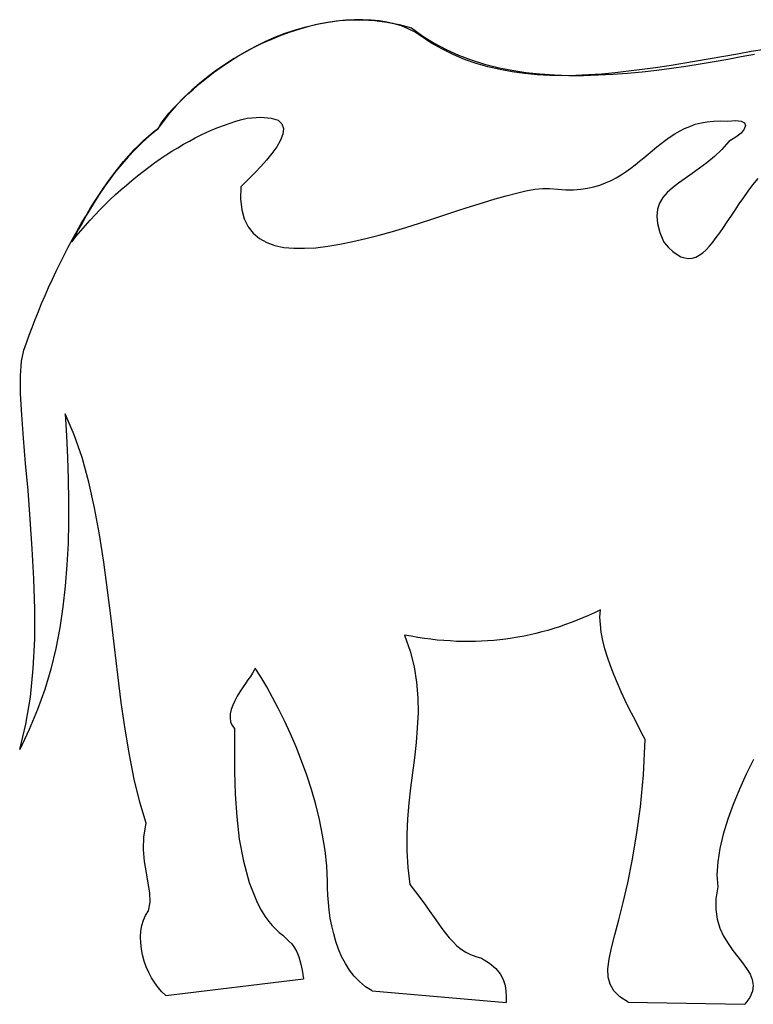
# Model space of a CAD drawing. Units: inches. Extents: x 386 to 107067, y -7 to 96314.
# Tile 9 of 10: x 107062.699 to 107064.862, y 96311.382 to 96314.283. Entities that reach past the tile are written whole.
import ezdxf

# ---------------------------------------------------------------- set-up
doc = ezdxf.new("R2010")
doc.units = ezdxf.units.IN
doc.layers.add('A-ELEV', color=7, linetype='Continuous', lineweight=25)
doc.layers.add('freecads.com', color=7, linetype='Continuous')

# ---------------------------------------------------------------- blocks, each defined once
blk = doc.blocks.new('elephant')
at = {"layer": 'freecads.com'}
for p, q in [((104457.3165, 95264.9791), (104457.3504, 95264.9835)), ((104457.3684, 95264.9845), (104457.3416, 95264.9818)), ((104457.3504, 95264.9835), (104457.3843, 95264.9856)), ((104457.3941, 95264.9862), (104457.3684, 95264.9845)), ((104457.3843, 95264.9856), (104457.4193, 95264.9856)), ((104457.4193, 95264.9862), (104457.3941, 95264.9862)), ((104457.4439, 95264.9851), (104457.4193, 95264.9862)), ((104457.4193, 95264.9856), (104457.4543, 95264.9835)), ((104457.4674, 95264.9829), (104457.4439, 95264.9851)), ((104457.4543, 95264.9835), (104457.4898, 95264.9791)), ((104457.4898, 95264.9791), (104457.4674, 95264.9829)), ((104457.1896, 95264.9463), (104457.2202, 95264.9567)), ((104457.2328, 95264.9583), (104457.2049, 95264.949)), ((104457.2202, 95264.9567), (104457.2514, 95264.9654)), ((104457.2601, 95264.966), (104457.2328, 95264.9583)), ((104457.2514, 95264.9654), (104457.2836, 95264.9731)), ((104457.288, 95264.9725), (104457.2601, 95264.966)), ((104457.2836, 95264.9731), (104457.3165, 95264.9791)), ((104457.3148, 95264.9774), (104457.288, 95264.9725)), ((104457.3416, 95264.9818), (104457.3148, 95264.9774)), ((104457.4898, 95264.9791), (104457.5259, 95264.972)), ((104457.5117, 95264.9742), (104457.4898, 95264.9791)), ((104457.5325, 95264.9676), (104457.5117, 95264.9742)), ((104457.5259, 95264.972), (104457.5625, 95264.9621)), ((104457.5522, 95264.9594), (104457.5325, 95264.9676)), ((104457.5708, 95264.9501), (104457.5522, 95264.9594)), ((104457.5625, 95264.9621), (104457.5954, 95264.9381)), ((104457.1491, 95264.9277), (104457.1212, 95264.9156)), ((104457.1311, 95264.9217), (104457.1595, 95264.9342)), ((104457.177, 95264.9392), (104457.1491, 95264.9277)), ((104457.1595, 95264.9342), (104457.1896, 95264.9463)), ((104457.2049, 95264.949), (104457.177, 95264.9392)), ((104457.5877, 95264.9392), (104457.5708, 95264.9501)), ((104457.6194, 95264.9184), (104457.5877, 95264.9392)), ((104457.5954, 95264.9381), (104457.6292, 95264.9167)), ((104457.0939, 95264.902), (104457.0665, 95264.8872)), ((104457.0758, 95264.8932), (104457.1032, 95264.908)), ((104457.1212, 95264.9156), (104457.0939, 95264.902)), ((104457.1032, 95264.908), (104457.1311, 95264.9217)), ((104457.6517, 95264.8998), (104457.6194, 95264.9184)), ((104457.6292, 95264.9167), (104457.6648, 95264.8981)), ((104457.685, 95264.8834), (104457.6517, 95264.8998)), ((104457.6648, 95264.8981), (104457.7009, 95264.8817)), ((104458.6048, 95264.8987), (104458.5644, 95264.8921)), ((104457.0398, 95264.8719), (104457.0135, 95264.8549)), ((104457.0255, 95264.8626), (104457.0501, 95264.8784)), ((104457.0665, 95264.8872), (104457.0398, 95264.8719)), ((104457.0501, 95264.8784), (104457.0758, 95264.8932)), ((104457.7184, 95264.8691), (104457.685, 95264.8834)), ((104457.7009, 95264.8817), (104457.7386, 95264.8675)), ((104457.7528, 95264.8571), (104457.7184, 95264.8691)), ((104457.7386, 95264.8675), (104457.7775, 95264.8555)), ((104458.443, 95264.8708), (104458.4025, 95264.8642)), ((104458.4834, 95264.8779), (104458.443, 95264.8708)), ((104458.4545, 95264.8631), (104458.4949, 95264.8702)), ((104458.5239, 95264.885), (104458.4834, 95264.8779)), ((104458.4949, 95264.8702), (104458.5348, 95264.8773)), ((104458.5644, 95264.8921), (104458.5239, 95264.885)), ((104458.5348, 95264.8773), (104458.5737, 95264.885)), ((104456.9878, 95264.8374), (104456.9626, 95264.8189)), ((104456.979, 95264.8303), (104457.0015, 95264.8467)), ((104457.0135, 95264.8549), (104456.9878, 95264.8374)), ((104457.0015, 95264.8467), (104457.0255, 95264.8626)), ((104457.7878, 95264.8473), (104457.7528, 95264.8571)), ((104457.7775, 95264.8555), (104457.8174, 95264.8451)), ((104457.8234, 95264.8391), (104457.7878, 95264.8473)), ((104457.8174, 95264.8451), (104457.8579, 95264.8374)), ((104457.8595, 95264.8325), (104457.8234, 95264.8391)), ((104457.8579, 95264.8374), (104457.8994, 95264.8309)), ((104458.2423, 95264.8391), (104458.2024, 95264.8342)), ((104458.2822, 95264.8446), (104458.2423, 95264.8391)), ((104458.2429, 95264.8325), (104458.286, 95264.8374)), ((104458.3221, 95264.8506), (104458.2822, 95264.8446)), ((104458.286, 95264.8374), (104458.3287, 95264.8435)), ((104458.3621, 95264.8571), (104458.3221, 95264.8506)), ((104458.3287, 95264.8435), (104458.3714, 95264.8495)), ((104458.4025, 95264.8642), (104458.3621, 95264.8571)), ((104458.3714, 95264.8495), (104458.4135, 95264.856)), ((104458.4135, 95264.856), (104458.4545, 95264.8631)), ((104456.9626, 95264.8189), (104456.938, 95264.7992)), ((104456.938, 95264.7981), (104456.9577, 95264.8139)), ((104456.9577, 95264.8139), (104456.979, 95264.8303)), ((104457.8961, 95264.8276), (104457.8595, 95264.8325)), ((104457.9328, 95264.8238), (104457.8961, 95264.8276)), ((104457.8994, 95264.8309), (104457.941, 95264.8265)), ((104457.9705, 95264.8221), (104457.9328, 95264.8238)), ((104457.941, 95264.8265), (104457.9836, 95264.8232)), ((104458.0082, 95264.821), (104457.9705, 95264.8221)), ((104457.9836, 95264.8232), (104458.0263, 95264.8221)), ((104458.0465, 95264.8216), (104458.0082, 95264.821)), ((104458.0263, 95264.8221), (104458.0695, 95264.8221)), ((104458.0848, 95264.8232), (104458.0465, 95264.8216)), ((104458.0695, 95264.8221), (104458.1127, 95264.8232)), ((104458.1236, 95264.826), (104458.0848, 95264.8232)), ((104458.1127, 95264.8232), (104458.1559, 95264.8254)), ((104458.163, 95264.8298), (104458.1236, 95264.826)), ((104458.1559, 95264.8254), (104458.1996, 95264.8287)), ((104458.2024, 95264.8342), (104458.163, 95264.8298)), ((104458.1996, 95264.8287), (104458.2429, 95264.8325)), ((104456.9019, 95264.7663), (104456.9194, 95264.7817)), ((104456.938, 95264.7992), (104456.9145, 95264.7784)), ((104456.9194, 95264.7817), (104456.938, 95264.7981)), ((104456.8915, 95264.757), (104456.8697, 95264.7341)), ((104456.8719, 95264.7368), (104456.8861, 95264.751)), ((104456.8861, 95264.751), (104456.9019, 95264.7663)), ((104456.9145, 95264.7784), (104456.8915, 95264.757)), ((104456.8472, 95264.7106), (104456.8587, 95264.7231)), ((104456.8697, 95264.7341), (104456.8489, 95264.7111)), ((104456.8587, 95264.7231), (104456.8719, 95264.7368)), ((104456.8489, 95264.7111), (104456.8297, 95264.6865)), ((104456.8297, 95264.6887), (104456.8379, 95264.6985)), ((104456.8379, 95264.6985), (104456.8472, 95264.7106)), ((104457.0447, 95264.6871), (104457.0616, 95264.692)), ((104457.0616, 95264.692), (104457.078, 95264.6958)), ((104457.078, 95264.6958), (104457.1185, 95264.6985)), ((104457.1185, 95264.6985), (104457.1486, 95264.6964)), ((104457.1486, 95264.6964), (104457.1688, 95264.6898)), ((104456.8013, 95264.6553), (104456.8161, 95264.6663)), ((104456.8297, 95264.6865), (104456.8111, 95264.6613)), ((104456.8161, 95264.6663), (104456.8188, 95264.6723)), ((104456.8188, 95264.6723), (104456.8232, 95264.6794)), ((104456.8232, 95264.6794), (104456.8297, 95264.6887)), ((104456.9768, 95264.6624), (104456.9938, 95264.6696)), ((104456.9938, 95264.6696), (104457.0108, 95264.6756)), ((104457.0108, 95264.6756), (104457.0277, 95264.6816)), ((104457.0277, 95264.6816), (104457.0447, 95264.6871)), ((104457.1688, 95264.6898), (104457.1803, 95264.6794)), ((104457.1803, 95264.6794), (104457.1852, 95264.6652)), ((104457.1852, 95264.6652), (104457.183, 95264.6493)), ((104458.3528, 95264.6581), (104458.3675, 95264.6652)), ((104458.3675, 95264.6652), (104458.3828, 95264.6717)), ((104458.3828, 95264.6717), (104458.3993, 95264.6778)), ((104458.3993, 95264.6778), (104458.4162, 95264.6821)), ((104458.4162, 95264.6821), (104458.4342, 95264.6854)), ((104458.4342, 95264.6854), (104458.4534, 95264.6876)), ((104458.4534, 95264.6876), (104458.473, 95264.6882)), ((104458.473, 95264.6882), (104458.4944, 95264.6871)), ((104458.4944, 95264.6871), (104458.5184, 95264.6892)), ((104458.5184, 95264.6892), (104458.5348, 95264.6876)), ((104458.5436, 95264.6635), (104458.5343, 95264.652)), ((104458.5348, 95264.6876), (104458.5447, 95264.6821)), ((104458.5474, 95264.6739), (104458.5436, 95264.6635)), ((104458.5447, 95264.6821), (104458.5474, 95264.6739)), ((104456.7887, 95264.6428), (104456.7669, 95264.6231)), ((104456.7718, 95264.6302), (104456.7865, 95264.6433)), ((104456.7865, 95264.6433), (104456.8013, 95264.6553)), ((104456.8111, 95264.6613), (104456.7887, 95264.6428)), ((104456.9074, 95264.6285), (104456.9249, 95264.6378)), ((104456.9249, 95264.6378), (104456.9424, 95264.6466)), ((104456.9424, 95264.6466), (104456.9593, 95264.6548)), ((104456.9593, 95264.6548), (104456.9768, 95264.6624)), ((104457.183, 95264.6493), (104457.1765, 95264.6313)), ((104458.3117, 95264.6313), (104458.3249, 95264.6411)), ((104458.3249, 95264.6411), (104458.3385, 95264.6499)), ((104458.3385, 95264.6499), (104458.3528, 95264.6581)), ((104458.5184, 95264.6395), (104458.4977, 95264.6274)), ((104458.5343, 95264.652), (104458.5184, 95264.6395)), ((104456.7422, 95264.6012), (104456.757, 95264.6159)), ((104456.7669, 95264.6231), (104456.7466, 95264.6028)), ((104456.757, 95264.6159), (104456.7718, 95264.6302)), ((104456.8554, 95264.5985), (104456.8729, 95264.6088)), ((104456.8729, 95264.6088), (104456.8905, 95264.6192)), ((104456.8905, 95264.6192), (104456.9074, 95264.6285)), ((104457.165, 95264.6116), (104457.1508, 95264.5919)), ((104457.1765, 95264.6313), (104457.165, 95264.6116)), ((104458.2729, 95264.6006), (104458.2855, 95264.611)), ((104458.2855, 95264.611), (104458.2986, 95264.6214)), ((104458.2986, 95264.6214), (104458.3117, 95264.6313)), ((104458.4977, 95264.6274), (104458.4774, 95264.6039)), ((104456.7269, 95264.5821), (104456.7083, 95264.5607)), ((104456.7133, 95264.5684), (104456.728, 95264.5848)), ((104456.7466, 95264.6028), (104456.7269, 95264.5821)), ((104456.728, 95264.5848), (104456.7422, 95264.6012)), ((104456.8046, 95264.564), (104456.8215, 95264.576)), ((104456.8215, 95264.576), (104456.8385, 95264.5875)), ((104456.8385, 95264.5875), (104456.8554, 95264.5985)), ((104457.1508, 95264.5919), (104457.1349, 95264.5722)), ((104458.2352, 95264.5689), (104458.2478, 95264.5793)), ((104458.2478, 95264.5793), (104458.2604, 95264.5903)), ((104458.2604, 95264.5903), (104458.2729, 95264.6006)), ((104458.4561, 95264.5831), (104458.4337, 95264.5646)), ((104458.4774, 95264.6039), (104458.4561, 95264.5831)), ((104456.6848, 95264.5317), (104456.699, 95264.5503)), ((104456.7083, 95264.5607), (104456.6908, 95264.5394)), ((104456.699, 95264.5503), (104456.7133, 95264.5684)), ((104456.7707, 95264.5389), (104456.7876, 95264.5514)), ((104456.7876, 95264.5514), (104456.8046, 95264.564)), ((104457.1179, 95264.5531), (104457.1015, 95264.5361)), ((104457.1349, 95264.5722), (104457.1179, 95264.5531)), ((104458.1953, 95264.5383), (104458.2089, 95264.5482)), ((104458.2089, 95264.5482), (104458.2221, 95264.5585)), ((104458.2221, 95264.5585), (104458.2352, 95264.5689)), ((104458.4118, 95264.5482), (104458.3905, 95264.5328)), ((104458.4337, 95264.5646), (104458.4118, 95264.5482)), ((104456.6701, 95264.5126), (104456.6848, 95264.5317)), ((104456.6908, 95264.5394), (104456.6739, 95264.5175)), ((104456.7379, 95264.5126), (104456.7543, 95264.5263)), ((104456.7543, 95264.5263), (104456.7707, 95264.5389)), ((104457.0862, 95264.5208), (104457.0736, 95264.5082)), ((104457.1015, 95264.5361), (104457.0862, 95264.5208)), ((104458.151, 95264.5126), (104458.1663, 95264.5203)), ((104458.1663, 95264.5203), (104458.181, 95264.529)), ((104458.181, 95264.529), (104458.1953, 95264.5383)), ((104458.3697, 95264.5186), (104458.35, 95264.5044)), ((104458.3905, 95264.5328), (104458.3697, 95264.5186)), ((104458.5693, 95264.4995), (104458.5846, 95264.5181)), ((104456.6422, 95264.4721), (104456.6564, 95264.4929)), ((104456.658, 95264.4956), (104456.6433, 95264.4738)), ((104456.6564, 95264.4929), (104456.6701, 95264.5126)), ((104456.6739, 95264.5175), (104456.658, 95264.4956)), ((104456.7056, 95264.4852), (104456.7215, 95264.4989)), ((104456.7215, 95264.4989), (104456.7379, 95264.5126)), ((104457.0594, 95264.494), (104457.0583, 95264.4579)), ((104457.0643, 95264.4989), (104457.0594, 95264.494)), ((104457.0736, 95264.5082), (104457.0643, 95264.4989)), ((104457.9257, 95264.4863), (104457.9486, 95264.4891)), ((104457.9486, 95264.4891), (104457.9689, 95264.4891)), ((104457.9689, 95264.4891), (104457.994, 95264.4863)), ((104458.0613, 95264.4863), (104458.081, 95264.4896)), ((104458.081, 95264.4896), (104458.1001, 95264.4935)), ((104458.1001, 95264.4935), (104458.1176, 95264.4989)), ((104458.1176, 95264.4989), (104458.1346, 95264.5055)), ((104458.1346, 95264.5055), (104458.151, 95264.5126)), ((104458.3325, 95264.4907), (104458.3167, 95264.4765)), ((104458.35, 95264.5044), (104458.3325, 95264.4907)), ((104458.5551, 95264.4809), (104458.5693, 95264.4995)), ((104456.6285, 95264.4513), (104456.6422, 95264.4721)), ((104456.6433, 95264.4738), (104456.6291, 95264.4519)), ((104456.6739, 95264.4563), (104456.6897, 95264.471)), ((104456.6897, 95264.471), (104456.7056, 95264.4852)), ((104457.8092, 95264.4579), (104457.8415, 95264.4672)), ((104457.8415, 95264.4672), (104457.8721, 95264.4754)), ((104457.8721, 95264.4754), (104457.8999, 95264.482)), ((104457.8999, 95264.482), (104457.9257, 95264.4863)), ((104457.994, 95264.4863), (104458.0175, 95264.4847)), ((104458.0175, 95264.4847), (104458.0399, 95264.4847)), ((104458.0399, 95264.4847), (104458.0613, 95264.4863)), ((104458.3035, 95264.4617), (104458.2937, 95264.4459)), ((104458.3167, 95264.4765), (104458.3035, 95264.4617)), ((104458.5288, 95264.4437), (104458.542, 95264.4623)), ((104458.542, 95264.4623), (104458.5551, 95264.4809)), ((104456.6148, 95264.4295), (104456.6285, 95264.4513)), ((104456.6291, 95264.4519), (104456.6159, 95264.43)), ((104456.6438, 95264.4262), (104456.6586, 95264.4415)), ((104456.6586, 95264.4415), (104456.6739, 95264.4563)), ((104457.0583, 95264.4579), (104457.0622, 95264.4262)), ((104457.702, 95264.4246), (104457.7392, 95264.4366)), ((104457.7392, 95264.4366), (104457.7747, 95264.4475)), ((104457.7747, 95264.4475), (104457.8092, 95264.4579)), ((104458.2937, 95264.4459), (104458.2877, 95264.4278)), ((104458.5168, 95264.4251), (104458.5288, 95264.4437)), ((104456.5886, 95264.3852), (104456.6017, 95264.4076)), ((104456.6033, 95264.4092), (104456.5919, 95264.3885)), ((104456.6017, 95264.4076), (104456.6148, 95264.4295)), ((104456.6159, 95264.43), (104456.6033, 95264.4092)), ((104456.6148, 95264.3956), (104456.6291, 95264.4109)), ((104456.6291, 95264.4109), (104456.6438, 95264.4262)), ((104457.0622, 95264.4262), (104457.0693, 95264.3989)), ((104457.6249, 95264.3994), (104457.6637, 95264.412)), ((104457.6637, 95264.412), (104457.702, 95264.4246)), ((104458.2877, 95264.4278), (104458.2855, 95264.4076)), ((104458.2855, 95264.4076), (104458.2877, 95264.3852)), ((104458.4933, 95264.3907), (104458.5048, 95264.4076)), ((104458.5048, 95264.4076), (104458.5168, 95264.4251)), ((104456.5754, 95264.3622), (104456.5886, 95264.3852)), ((104456.5919, 95264.3885), (104456.5809, 95264.3688)), ((104456.5869, 95264.3638), (104456.6006, 95264.3797)), ((104456.6006, 95264.3797), (104456.6148, 95264.3956)), ((104457.0693, 95264.3989), (104457.0807, 95264.3759)), ((104457.0807, 95264.3759), (104457.0955, 95264.3567)), ((104457.5062, 95264.3622), (104457.5461, 95264.3742)), ((104457.5461, 95264.3742), (104457.5855, 95264.3868)), ((104457.5855, 95264.3868), (104457.6249, 95264.3994)), ((104458.2877, 95264.3852), (104458.2942, 95264.3595)), ((104458.4714, 95264.3584), (104458.4823, 95264.3742)), ((104458.4823, 95264.3742), (104458.4933, 95264.3907)), ((104456.5705, 95264.3496), (104456.5607, 95264.3316)), ((104456.5607, 95264.3316), (104456.5738, 95264.348)), ((104456.5629, 95264.3392), (104456.5754, 95264.3622)), ((104456.5809, 95264.3688), (104456.5705, 95264.3496)), ((104456.5738, 95264.348), (104456.5869, 95264.3638)), ((104457.0955, 95264.3567), (104457.1141, 95264.3414)), ((104457.4275, 95264.3409), (104457.4668, 95264.3513)), ((104457.4668, 95264.3513), (104457.5062, 95264.3622)), ((104458.2942, 95264.3595), (104458.3068, 95264.3305)), ((104458.4512, 95264.3305), (104458.461, 95264.3442)), ((104458.461, 95264.3442), (104458.4714, 95264.3584)), ((104456.5383, 95264.2922), (104456.5503, 95264.3157)), ((104456.5503, 95264.3157), (104456.5629, 95264.3392)), ((104457.1141, 95264.3414), (104457.1354, 95264.3294)), ((104457.1354, 95264.3294), (104457.1595, 95264.3212)), ((104457.1595, 95264.3212), (104457.1863, 95264.3152)), ((104457.1863, 95264.3152), (104457.2158, 95264.3124)), ((104457.2804, 95264.3141), (104457.3154, 95264.3185)), ((104457.3154, 95264.3185), (104457.3514, 95264.3245)), ((104457.3514, 95264.3245), (104457.3892, 95264.3321)), ((104457.3892, 95264.3321), (104457.4275, 95264.3409)), ((104458.3068, 95264.3305), (104458.3205, 95264.3152)), ((104458.3205, 95264.3152), (104458.3331, 95264.3032)), ((104458.431, 95264.3081), (104458.4408, 95264.3185)), ((104458.4408, 95264.3185), (104458.4512, 95264.3305)), ((104456.5262, 95264.2687), (104456.5383, 95264.2922)), ((104457.2158, 95264.3124), (104457.247, 95264.3124)), ((104457.247, 95264.3124), (104457.2804, 95264.3141)), ((104458.3331, 95264.3032), (104458.3457, 95264.2939)), ((104458.3457, 95264.2939), (104458.3571, 95264.2878)), ((104458.3571, 95264.2878), (104458.3686, 95264.284)), ((104458.3905, 95264.2835), (104458.4009, 95264.2868)), ((104458.4009, 95264.2868), (104458.4107, 95264.2922)), ((104458.4107, 95264.2922), (104458.4211, 95264.2993)), ((104458.4211, 95264.2993), (104458.431, 95264.3081)), ((104456.5148, 95264.2446), (104456.5262, 95264.2687)), ((104458.3686, 95264.284), (104458.3796, 95264.2824)), ((104458.3796, 95264.2824), (104458.3905, 95264.2835)), ((104456.5033, 95264.2211), (104456.5148, 95264.2446)), ((104456.4923, 95264.197), (104456.5033, 95264.2211)), ((104456.4716, 95264.1495), (104456.4819, 95264.173)), ((104456.4819, 95264.173), (104456.4923, 95264.197)), ((104456.4623, 95264.126), (104456.4716, 95264.1495)), ((104456.4524, 95264.1024), (104456.4623, 95264.126)), ((104456.4437, 95264.0795), (104456.4524, 95264.1024)), ((104456.4272, 95264.0341), (104456.4354, 95264.0565)), ((104456.4354, 95264.0565), (104456.4437, 95264.0795)), ((104456.4196, 95264.0122), (104456.4272, 95264.0341)), ((104456.4125, 95263.98), (104456.4196, 95264.0122)), ((104456.4097, 95263.9367), (104456.4125, 95263.98)), ((104456.4097, 95263.8837), (104456.4097, 95263.9367)), ((104456.413, 95263.8219), (104456.4097, 95263.8837)), ((104456.4179, 95263.753), (104456.413, 95263.8219)), ((104456.5678, 95263.7629), (104456.5415, 95263.8246)), ((104456.5415, 95263.8246), (104456.5448, 95263.7601)), ((104456.4245, 95263.6781), (104456.4179, 95263.753)), ((104456.5448, 95263.7601), (104456.5481, 95263.6961)), ((104456.5908, 95263.6956), (104456.5678, 95263.7629)), ((104456.4316, 95263.5983), (104456.4245, 95263.6781)), ((104456.5481, 95263.6961), (104456.5497, 95263.6322)), ((104456.6105, 95263.6234), (104456.5908, 95263.6956)), ((104456.5497, 95263.6322), (104456.5514, 95263.5687)), ((104456.6274, 95263.5474), (104456.6105, 95263.6234)), ((104456.4382, 95263.514), (104456.4316, 95263.5983)), ((104456.5514, 95263.5687), (104456.5514, 95263.5053)), ((104456.6422, 95263.4686), (104456.6274, 95263.5474)), ((104456.4442, 95263.4271), (104456.4382, 95263.514)), ((104456.5514, 95263.5053), (104456.5497, 95263.4424)), ((104456.6547, 95263.3877), (104456.6422, 95263.4686)), ((104456.4491, 95263.3385), (104456.4442, 95263.4271)), ((104456.5497, 95263.4424), (104456.5465, 95263.3795)), ((104456.6662, 95263.3046), (104456.6547, 95263.3877)), ((104456.5465, 95263.3795), (104456.5415, 95263.3172)), ((104456.4513, 95263.2494), (104456.4491, 95263.3385)), ((104456.5415, 95263.3172), (104456.5344, 95263.2554)), ((104456.6766, 95263.2215), (104456.6662, 95263.3046)), ((104456.4513, 95263.1608), (104456.4513, 95263.2494)), ((104456.5344, 95263.2554), (104456.5251, 95263.1936)), ((104458.1193, 95263.2466), (104458.1023, 95263.2384)), ((104458.1182, 95263.2258), (104458.1193, 95263.2466)), ((104456.6865, 95263.1378), (104456.6766, 95263.2215)), ((104458.0509, 95263.2165), (104458.0334, 95263.2094)), ((104458.0678, 95263.2231), (104458.0509, 95263.2165)), ((104458.0848, 95263.2308), (104458.0678, 95263.2231)), ((104458.1023, 95263.2384), (104458.0848, 95263.2308)), ((104458.1193, 95263.204), (104458.1182, 95263.2258)), ((104456.5251, 95263.1936), (104456.5131, 95263.1329)), ((104457.9645, 95263.1865), (104457.947, 95263.1821)), ((104457.982, 95263.1919), (104457.9645, 95263.1865)), ((104457.9989, 95263.1974), (104457.982, 95263.1919)), ((104458.0164, 95263.2034), (104457.9989, 95263.1974)), ((104458.0334, 95263.2094), (104458.0164, 95263.2034)), ((104458.122, 95263.181), (104458.1193, 95263.204)), ((104456.4469, 95263.0738), (104456.4513, 95263.1608)), ((104457.5615, 95263.169), (104457.5418, 95263.1728)), ((104457.5418, 95263.1728), (104457.5582, 95263.1252)), ((104457.5806, 95263.1657), (104457.5615, 95263.169)), ((104457.6003, 95263.163), (104457.5806, 95263.1657)), ((104457.6194, 95263.1602), (104457.6003, 95263.163)), ((104457.6385, 95263.158), (104457.6194, 95263.1602)), ((104457.6577, 95263.1564), (104457.6385, 95263.158)), ((104457.6763, 95263.1553), (104457.6577, 95263.1564)), ((104457.6949, 95263.1542), (104457.6763, 95263.1553)), ((104457.7135, 95263.1537), (104457.6949, 95263.1542)), ((104457.7687, 95263.1548), (104457.7507, 95263.1537)), ((104457.7868, 95263.1553), (104457.7687, 95263.1548)), ((104457.8048, 95263.157), (104457.7868, 95263.1553)), ((104457.8229, 95263.1586), (104457.8048, 95263.157)), ((104457.8409, 95263.1608), (104457.8229, 95263.1586)), ((104457.859, 95263.1635), (104457.8409, 95263.1608)), ((104457.8764, 95263.1662), (104457.859, 95263.1635)), ((104457.8945, 95263.1695), (104457.8764, 95263.1662)), ((104457.912, 95263.1734), (104457.8945, 95263.1695)), ((104457.9295, 95263.1772), (104457.912, 95263.1734)), ((104457.947, 95263.1821), (104457.9295, 95263.1772)), ((104458.1264, 95263.157), (104458.122, 95263.181)), ((104458.1329, 95263.1323), (104458.1264, 95263.157)), ((104456.5131, 95263.1329), (104456.4984, 95263.0722)), ((104456.6968, 95263.0552), (104456.6865, 95263.1378)), ((104457.5582, 95263.1252), (104457.5702, 95263.0787)), ((104457.7321, 95263.1537), (104457.7135, 95263.1537)), ((104457.7507, 95263.1537), (104457.7321, 95263.1537)), ((104458.1406, 95263.1077), (104458.1329, 95263.1323)), ((104458.1493, 95263.082), (104458.1406, 95263.1077)), ((104456.4387, 95262.9901), (104456.4469, 95263.0738)), ((104456.4984, 95263.0722), (104456.4808, 95263.012)), ((104457.0982, 95263.0689), (104457.0933, 95263.0607)), ((104457.1015, 95263.0754), (104457.0982, 95263.0689)), ((104457.1179, 95263.0492), (104457.1015, 95263.0754)), ((104457.5702, 95263.0787), (104457.5773, 95263.0334)), ((104458.1592, 95263.0569), (104458.1493, 95263.082)), ((104456.7067, 95262.9743), (104456.6968, 95263.0552)), ((104457.0802, 95263.0405), (104457.0725, 95263.0295)), ((104457.0873, 95263.0508), (104457.0802, 95263.0405)), ((104457.0933, 95263.0607), (104457.0873, 95263.0508)), ((104457.1354, 95263.0202), (104457.1179, 95263.0492)), ((104458.1696, 95263.0312), (104458.1592, 95263.0569)), ((104456.4808, 95263.012), (104456.4595, 95262.953)), ((104457.0643, 95263.0175), (104457.0561, 95263.0049)), ((104457.0725, 95263.0295), (104457.0643, 95263.0175)), ((104457.1529, 95262.9891), (104457.1354, 95263.0202)), ((104457.5773, 95263.0334), (104457.5811, 95262.988)), ((104458.181, 95263.0055), (104458.1696, 95263.0312)), ((104456.4256, 95262.9103), (104456.4387, 95262.9901)), ((104457.0485, 95262.9923), (104457.0414, 95262.9792)), ((104457.0561, 95263.0049), (104457.0485, 95262.9923)), ((104457.1704, 95262.9551), (104457.1529, 95262.9891)), ((104457.5811, 95262.988), (104457.5817, 95262.9437)), ((104458.1925, 95262.9803), (104458.181, 95263.0055)), ((104458.2046, 95262.9557), (104458.1925, 95262.9803)), ((104456.4595, 95262.953), (104456.4354, 95262.8939)), ((104456.7182, 95262.895), (104456.7067, 95262.9743)), ((104457.031, 95262.953), (104457.0277, 95262.9404)), ((104457.0354, 95262.9661), (104457.031, 95262.953)), ((104457.0414, 95262.9792), (104457.0354, 95262.9661)), ((104457.1879, 95262.9196), (104457.1704, 95262.9551)), ((104458.2166, 95262.9316), (104458.2046, 95262.9557)), ((104457.0277, 95262.9404), (104457.0272, 95262.9283)), ((104457.0272, 95262.9283), (104457.0288, 95262.9174)), ((104457.5817, 95262.9437), (104457.5795, 95262.8994)), ((104458.2286, 95262.9087), (104458.2166, 95262.9316)), ((104456.407, 95262.8359), (104456.4256, 95262.9103)), ((104456.4354, 95262.8939), (104456.407, 95262.8359)), ((104456.7308, 95262.8195), (104456.7182, 95262.895)), ((104457.0288, 95262.9174), (104457.0332, 95262.9065)), ((104457.0332, 95262.9065), (104457.0403, 95262.8972)), ((104457.0403, 95262.8972), (104457.0403, 95262.8348)), ((104457.2054, 95262.8819), (104457.1879, 95262.9196)), ((104457.5795, 95262.8994), (104457.5762, 95262.8556)), ((104458.2401, 95262.8863), (104458.2286, 95262.9087)), ((104457.2224, 95262.843), (104457.2054, 95262.8819)), ((104458.2516, 95262.8649), (104458.2401, 95262.8863)), ((104458.2461, 95262.7605), (104458.2516, 95262.8649)), ((104457.0403, 95262.8348), (104457.0408, 95262.7703)), ((104457.2382, 95262.802), (104457.2224, 95262.843)), ((104457.5762, 95262.8556), (104457.5713, 95262.8113)), ((104456.7444, 95262.7479), (104456.7308, 95262.8195)), ((104457.5713, 95262.8113), (104457.5653, 95262.767)), ((104458.571, 95262.8058), (104458.5496, 95262.7627)), ((104457.2536, 95262.7599), (104457.2382, 95262.802)), ((104456.7608, 95262.6806), (104456.7444, 95262.7479)), ((104457.0408, 95262.7703), (104457.0425, 95262.7041)), ((104457.2672, 95262.7173), (104457.2536, 95262.7599)), ((104457.5653, 95262.767), (104457.5598, 95262.7227)), ((104458.2374, 95262.6664), (104458.2461, 95262.7605)), ((104458.5496, 95262.7627), (104458.5294, 95262.7184)), ((104457.5598, 95262.7227), (104457.5543, 95262.6773)), ((104457.0425, 95262.7041), (104457.0469, 95262.6374)), ((104457.2798, 95262.673), (104457.2672, 95262.7173)), ((104458.5294, 95262.7184), (104458.5113, 95262.6735)), ((104456.78, 95262.6188), (104456.7608, 95262.6806)), ((104457.2913, 95262.6287), (104457.2798, 95262.673)), ((104457.5543, 95262.6773), (104457.5505, 95262.6314)), ((104458.2259, 95262.5827), (104458.2374, 95262.6664)), ((104458.5113, 95262.6735), (104458.4955, 95262.6298)), ((104457.0469, 95262.6374), (104457.0545, 95262.5712)), ((104456.7729, 95262.5784), (104456.78, 95262.6188)), ((104457.3001, 95262.5833), (104457.2913, 95262.6287)), ((104457.5505, 95262.6314), (104457.5483, 95262.5849)), ((104458.4955, 95262.6298), (104458.4818, 95262.586)), ((104456.7718, 95262.5406), (104456.7729, 95262.5784)), ((104457.3077, 95262.5379), (104457.3001, 95262.5833)), ((104457.5483, 95262.5849), (104457.5483, 95262.5368)), ((104458.2133, 95262.5078), (104458.2259, 95262.5827)), ((104458.4818, 95262.586), (104458.472, 95262.5439)), ((104457.0545, 95262.5712), (104457.0665, 95262.5062)), ((104456.7751, 95262.5051), (104456.7718, 95262.5406)), ((104457.3126, 95262.4925), (104457.3077, 95262.5379)), ((104457.5483, 95262.5368), (104457.5511, 95262.4876)), ((104458.472, 95262.5439), (104458.4654, 95262.504)), ((104456.7805, 95262.4723), (104456.7751, 95262.5051)), ((104457.0665, 95262.5062), (104457.084, 95262.4433)), ((104457.3148, 95262.4471), (104457.3126, 95262.4925)), ((104457.5511, 95262.4876), (104457.5576, 95262.4373)), ((104458.2002, 95262.4422), (104458.2133, 95262.5078)), ((104458.4654, 95262.504), (104458.4632, 95262.4663)), ((104456.786, 95262.4416), (104456.7805, 95262.4723)), ((104458.4632, 95262.4663), (104458.4654, 95262.4312)), ((104456.7904, 95262.4127), (104456.786, 95262.4416)), ((104457.084, 95262.4433), (104457.1075, 95262.3842)), ((104457.3148, 95262.4274), (104457.3148, 95262.4471)), ((104457.5576, 95262.4373), (104457.5746, 95262.4159)), ((104458.1865, 95262.3842), (104458.2002, 95262.4422)), ((104458.4654, 95262.4312), (104458.4599, 95262.3957)), ((104456.7915, 95262.3853), (104456.7904, 95262.4127)), ((104457.3159, 95262.4061), (104457.3148, 95262.4274)), ((104457.3176, 95262.3842), (104457.3159, 95262.4061)), ((104457.5746, 95262.4159), (104457.5899, 95262.3957)), ((104456.7865, 95262.3596), (104456.7915, 95262.3853)), ((104457.1075, 95262.3842), (104457.119, 95262.3623)), ((104457.3197, 95262.3618), (104457.3176, 95262.3842)), ((104457.5899, 95262.3957), (104457.6041, 95262.3766)), ((104457.6041, 95262.3766), (104457.6167, 95262.358)), ((104458.1734, 95262.3334), (104458.1865, 95262.3842)), ((104458.4599, 95262.3957), (104458.4594, 95262.364)), ((104456.7718, 95262.3323), (104456.7783, 95262.3465)), ((104456.7783, 95262.3465), (104456.7865, 95262.3596)), ((104457.119, 95262.3623), (104457.13, 95262.3443)), ((104457.13, 95262.3443), (104457.1415, 95262.329)), ((104457.323, 95262.3388), (104457.3197, 95262.3618)), ((104457.6167, 95262.358), (104457.6292, 95262.3405)), ((104458.4594, 95262.364), (104458.4638, 95262.335)), ((104456.7647, 95262.3005), (104456.7674, 95262.317)), ((104456.7674, 95262.317), (104456.7718, 95262.3323)), ((104457.1415, 95262.329), (104457.1519, 95262.3164)), ((104457.1519, 95262.3164), (104457.1628, 95262.3055)), ((104457.3274, 95262.3153), (104457.323, 95262.3388)), ((104457.3329, 95262.2923), (104457.3274, 95262.3153)), ((104457.6292, 95262.3405), (104457.6407, 95262.3241)), ((104457.6407, 95262.3241), (104457.6517, 95262.3082)), ((104458.1619, 95262.2896), (104458.1734, 95262.3334)), ((104458.4638, 95262.335), (104458.472, 95262.3088)), ((104456.7636, 95262.283), (104456.7647, 95262.3005)), ((104457.1628, 95262.3055), (104457.1726, 95262.2962)), ((104457.1726, 95262.2962), (104457.1825, 95262.288)), ((104457.1825, 95262.288), (104457.1923, 95262.2798)), ((104457.3394, 95262.2694), (104457.3329, 95262.2923)), ((104457.6517, 95262.3082), (104457.6626, 95262.294)), ((104457.6626, 95262.294), (104457.6736, 95262.2803)), ((104458.1521, 95262.2513), (104458.1619, 95262.2896)), ((104458.472, 95262.3088), (104458.4829, 95262.2852)), ((104458.4829, 95262.2852), (104458.496, 95262.2634)), ((104456.7641, 95262.2655), (104456.7636, 95262.283)), ((104456.7658, 95262.2475), (104456.7641, 95262.2655)), ((104457.1923, 95262.2798), (104457.2011, 95262.271)), ((104457.2011, 95262.271), (104457.2093, 95262.2623)), ((104457.2093, 95262.2623), (104457.2169, 95262.2513)), ((104457.3476, 95262.247), (104457.3394, 95262.2694)), ((104457.6736, 95262.2803), (104457.685, 95262.2683)), ((104457.685, 95262.2683), (104457.6965, 95262.2573)), ((104457.6965, 95262.2573), (104457.7086, 95262.247)), ((104458.496, 95262.2634), (104458.5102, 95262.2431)), ((104456.7696, 95262.23), (104456.7658, 95262.2475)), ((104456.774, 95262.212), (104456.7696, 95262.23)), ((104457.2169, 95262.2513), (104457.224, 95262.2393)), ((104457.224, 95262.2393), (104457.23, 95262.2245)), ((104457.3564, 95262.2256), (104457.3476, 95262.247)), ((104457.3673, 95262.2049), (104457.3564, 95262.2256)), ((104457.7086, 95262.247), (104457.7222, 95262.2382)), ((104457.7222, 95262.2382), (104457.7364, 95262.2311)), ((104457.7364, 95262.2311), (104457.7518, 95262.2251)), ((104458.1455, 95262.218), (104458.1521, 95262.2513)), ((104458.5102, 95262.2431), (104458.5245, 95262.2245)), ((104456.78, 95262.195), (104456.774, 95262.212)), ((104457.23, 95262.2245), (104457.2355, 95262.2065)), ((104457.2355, 95262.2065), (104457.2399, 95262.1852)), ((104457.3799, 95262.1852), (104457.3673, 95262.2049)), ((104457.7518, 95262.2251), (104457.7687, 95262.2202)), ((104457.7687, 95262.2202), (104457.7928, 95262.206)), ((104457.7928, 95262.206), (104457.8108, 95262.1901)), ((104458.1417, 95262.1895), (104458.1455, 95262.218)), ((104458.5245, 95262.2245), (104458.5381, 95262.207)), ((104458.5381, 95262.207), (104458.5507, 95262.1901)), ((104456.7876, 95262.1781), (104456.78, 95262.195)), ((104456.7958, 95262.1622), (104456.7876, 95262.1781)), ((104457.2399, 95262.1852), (104457.2437, 95262.1595)), ((104457.3936, 95262.1671), (104457.3799, 95262.1852)), ((104457.8108, 95262.1901), (104457.8239, 95262.1742)), ((104457.8239, 95262.1742), (104457.8327, 95262.1573)), ((104458.1422, 95262.1649), (104458.1417, 95262.1895)), ((104458.5507, 95262.1901), (104458.5606, 95262.1737)), ((104458.5606, 95262.1737), (104458.5671, 95262.1573)), ((104456.8051, 95262.1474), (104456.7958, 95262.1622)), ((104456.815, 95262.1337), (104456.8051, 95262.1474)), ((104456.8379, 95262.1108), (104457.2437, 95262.1595)), ((104457.4094, 95262.1513), (104457.3936, 95262.1671)), ((104457.4269, 95262.1365), (104457.4094, 95262.1513)), ((104457.8327, 95262.1573), (104457.8382, 95262.1398)), ((104457.8382, 95262.1398), (104457.8404, 95262.1228)), ((104458.1482, 95262.1436), (104458.1422, 95262.1649)), ((104458.1592, 95262.1244), (104458.1482, 95262.1436)), ((104458.5671, 95262.1573), (104458.5699, 95262.1403)), ((104458.5699, 95262.1403), (104458.5677, 95262.1228)), ((104456.8259, 95262.1212), (104456.815, 95262.1337)), ((104456.8379, 95262.1108), (104456.8259, 95262.1212)), ((104457.4466, 95262.1244), (104457.4269, 95262.1365)), ((104457.4466, 95262.1244), (104457.8415, 95262.0895)), ((104457.8404, 95262.1228), (104457.8415, 95262.1059)), ((104458.1767, 95262.107), (104458.1592, 95262.1244)), ((104458.5677, 95262.1228), (104458.56, 95262.1042)), ((104457.8415, 95262.1059), (104457.8415, 95262.0895)), ((104458.2013, 95262.0911), (104458.1767, 95262.107)), ((104458.2013, 95262.0911), (104458.5452, 95262.0845)), ((104458.56, 95262.1042), (104458.5452, 95262.0845))]:
    blk.add_line(p, q, dxfattribs=at)

msp = doc.modelspace()

# ---------------------------------------------------------------- block references
at = {"layer": 'A-ELEV'}
msp.add_blockref('elephant', (2606.2918, 1049.297), dxfattribs=at)

doc.saveas('drawing.dxf')
